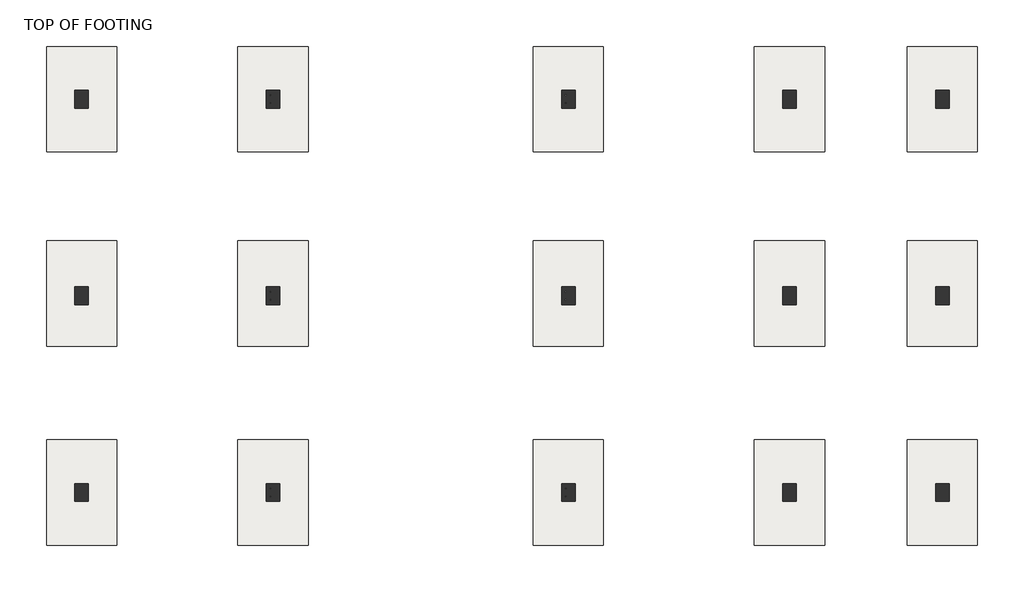
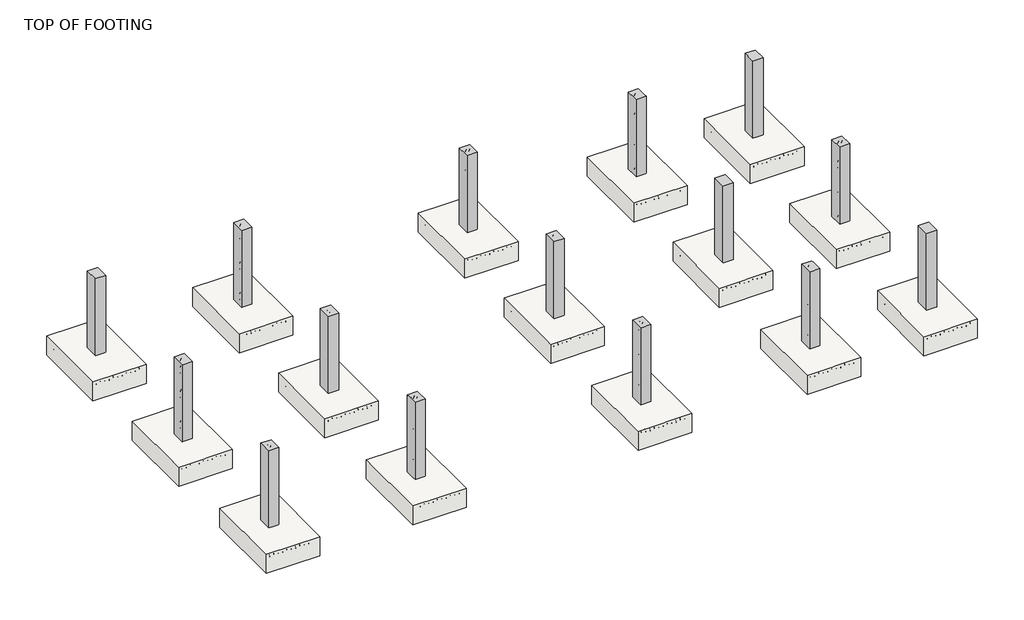
# One storey, part 1 of 8: 15 columns, 15 slabs.
"""IFC4 building model written with IfcOpenShell, lengths in millimetres."""

from ifc_helpers import new_model, si_unit, origin, place, context, project, spatial, faceted_brep, transform, mapped, element, save
from components import m_footing_rectangular_1800_x_1200_x_450mm_16ba7ea5

model = new_model("IFC4")

# Units and contexts
model_context = context("Model", 3, world=origin())
ifc_project = project(units=[si_unit("LENGTHUNIT", "METRE", prefix="MILLI")], contexts=[model_context])

# Site, building, storey
site = spatial("IfcSite", under=ifc_project)
building = spatial("IfcBuilding", under=site)
storey = spatial("IfcBuildingStorey", under=building, Name="TOP OF FOOTING", Elevation=-1828.8)

# Columns
placement = place(None, origin())
element("IfcColumn", 1, ObjectType="M_Concrete-Rectangular-Column : 9\" X 1' COLUMNS", at=placement, inside=storey, context=model_context, shape_type="Brep", body=[
    faceted_brep([(9617.8931183, 9077.6765586, -1828.8), (9617.8931183, 8772.8765586, -1828.8), (9389.2931183, 8772.8765586, -1828.8), (9389.2931183, 9077.6765586, -1828.8), (9617.8931183, 9077.6765586, 0.0), (9617.8931183, 8772.8765586, 0.0), (9389.2931183, 8772.8765586, 0.0), (9389.2931183, 8849.0765586, 0.0), (9389.2931183, 9077.6765586, 0.0)], [[[0, 1, 2, 3]], [[4, 5, 1, 0]], [[5, 6, 2, 1]], [[6, 7, 8, 3, 2]], [[8, 4, 0, 3]], [[4, 8, 7, 6, 5]]]),
])
element("IfcColumn", 2, ObjectType="M_Concrete-Rectangular-Column : 9\" X 1' COLUMNS", at=placement, inside=storey, context=model_context, shape_type="Brep", body=[
    faceted_brep([(9617.8931183, 5712.0180792, -1828.8), (9617.8931183, 5407.2180792, -1828.8), (9389.2931183, 5407.2180792, -1828.8), (9389.2931183, 5712.0180792, -1828.8), (9617.8931183, 5712.0180792, 0.0), (9617.8931183, 5407.2180792, 0.0), (9389.2931183, 5407.2180792, 0.0), (9389.2931183, 5445.3180792, 0.0), (9389.2931183, 5673.9180792, 0.0), (9389.2931183, 5712.0180792, 0.0)], [[[0, 1, 2, 3]], [[4, 5, 1, 0]], [[5, 6, 2, 1]], [[6, 7, 8, 9, 3, 2]], [[9, 4, 0, 3]], [[4, 9, 8, 7, 6, 5]]]),
])
element("IfcColumn", 3, ObjectType="M_Concrete-Rectangular-Column : 9\" X 1' COLUMNS", at=placement, inside=storey, context=model_context, shape_type="Brep", body=[
    faceted_brep([(9617.8931183, 2346.6765586, -1828.8), (9617.8931183, 2041.8765586, -1828.8), (9389.2931183, 2041.8765586, -1828.8), (9389.2931183, 2346.6765586, -1828.8), (9617.8931183, 2346.6765586, 0.0), (9617.8931183, 2041.8765586, 0.0), (9389.2931183, 2041.8765586, 0.0), (9389.2931183, 2270.4765586, 0.0), (9389.2931183, 2346.6765586, 0.0)], [[[0, 1, 2, 3]], [[4, 5, 1, 0]], [[5, 6, 2, 1]], [[6, 7, 8, 3, 2]], [[8, 4, 0, 3]], [[4, 8, 7, 6, 5]]]),
])
element("IfcColumn", 4, ObjectType="M_Concrete-Rectangular-Column : 9\" X 1' COLUMNS", at=placement, inside=storey, context=model_context, shape_type="Brep", body=[
    faceted_brep([(7001.6931183, 9077.6765586, -1828.8), (7001.6931183, 8772.8765586, -1828.8), (6773.0931183, 8772.8765586, -1828.8), (6773.0931183, 9077.6765586, -1828.8), (7001.6931183, 9077.6765586, 0.0), (7001.6931183, 8849.0765586, 0.0), (7001.6931183, 8772.8765586, 0.0), (7001.6931183, 8772.8765586, -300.0), (6773.0931183, 8772.8765586, 0.0), (6773.0931183, 8772.8765586, -300.0), (6773.0931183, 8849.0765586, 0.0), (6773.0931183, 9077.6765586, 0.0)], [[[0, 1, 2, 3]], [[1, 0, 4, 5, 6, 7]], [[2, 1, 7, 6, 8, 9]], [[3, 2, 9, 8, 10, 11]], [[0, 3, 11, 4]], [[8, 6, 5, 4, 11, 10]]]),
])
element("IfcColumn", 5, ObjectType="M_Concrete-Rectangular-Column : 9\" X 1' COLUMNS", at=placement, inside=storey, context=model_context, shape_type="Brep", body=[
    faceted_brep([(7001.6931183, 5712.0180792, -1828.8), (7001.6931183, 5407.2180792, -1828.8), (6773.0931183, 5407.2180792, -1828.8), (6773.0931183, 5712.0180792, -1828.8), (7001.6931183, 5712.0180792, -300.0), (7001.6931183, 5712.0180792, 0.0), (7001.6931183, 5673.9180792, 0.0), (7001.6931183, 5445.3180792, 0.0), (7001.6931183, 5407.2180792, 0.0), (7001.6931183, 5407.2180792, -300.0), (6773.0931183, 5407.2180792, 0.0), (6773.0931183, 5407.2180792, -300.0), (6773.0931183, 5445.3180792, 0.0), (6773.0931183, 5673.9180792, 0.0), (6773.0931183, 5712.0180792, 0.0), (6773.0931183, 5712.0180792, -300.0)], [[[0, 1, 2, 3]], [[1, 0, 4, 5, 6, 7, 8, 9]], [[2, 1, 9, 8, 10, 11]], [[3, 2, 11, 10, 12, 13, 14, 15]], [[0, 3, 15, 14, 5, 4]], [[10, 8, 7, 6, 5, 14, 13, 12]]]),
])
element("IfcColumn", 6, ObjectType="M_Concrete-Rectangular-Column : 9\" X 1' COLUMNS", at=placement, inside=storey, context=model_context, shape_type="Brep", body=[
    faceted_brep([(7001.6931183, 2346.6765586, -1828.8), (7001.6931183, 2041.8765586, -1828.8), (6773.0931183, 2041.8765586, -1828.8), (6773.0931183, 2346.6765586, -1828.8), (7001.6931183, 2346.6765586, -300.0), (7001.6931183, 2346.6765586, 0.0), (7001.6931183, 2270.4765586, 0.0), (7001.6931183, 2041.8765586, 0.0), (6773.0931183, 2041.8765586, 0.0), (6773.0931183, 2270.4765586, 0.0), (6773.0931183, 2346.6765586, 0.0), (6773.0931183, 2346.6765586, -300.0)], [[[0, 1, 2, 3]], [[1, 0, 4, 5, 6, 7]], [[2, 1, 7, 8]], [[3, 2, 8, 9, 10, 11]], [[0, 3, 11, 10, 5, 4]], [[8, 7, 6, 5, 10, 9]]]),
])
element("IfcColumn", 7, ObjectType="M_Concrete-Rectangular-Column : 9\" X 1' COLUMNS", at=placement, inside=storey, context=model_context, shape_type="Brep", body=[
    faceted_brep([(3217.0931183, 9077.6765586, -1828.8), (3217.0931183, 8772.8765586, -1828.8), (2988.4931183, 8772.8765586, -1828.8), (2988.4931183, 9077.6765586, -1828.8), (3217.0931183, 9077.6765586, 0.0), (3217.0931183, 8849.0765586, 0.0), (3217.0931183, 8772.8765586, 0.0), (3217.0931183, 8772.8765586, -300.0), (2988.4931183, 8772.8765586, 0.0), (2988.4931183, 8772.8765586, -300.0), (2988.4931183, 8849.0765586, 0.0), (2988.4931183, 9077.6765586, 0.0)], [[[0, 1, 2, 3]], [[1, 0, 4, 5, 6, 7]], [[2, 1, 7, 6, 8, 9]], [[3, 2, 9, 8, 10, 11]], [[0, 3, 11, 4]], [[8, 6, 5, 4, 11, 10]]]),
])
element("IfcColumn", 8, ObjectType="M_Concrete-Rectangular-Column : 9\" X 1' COLUMNS", at=placement, inside=storey, context=model_context, shape_type="Brep", body=[
    faceted_brep([(3217.0931183, 5712.0180792, -1828.8), (3217.0931183, 5407.2180792, -1828.8), (2988.4931183, 5407.2180792, -1828.8), (2988.4931183, 5712.0180792, -1828.8), (3217.0931183, 5712.0180792, -300.0), (3217.0931183, 5712.0180792, 0.0), (3217.0931183, 5673.9180792, 0.0), (3217.0931183, 5445.3180792, 0.0), (3217.0931183, 5407.2180792, 0.0), (3217.0931183, 5407.2180792, -300.0), (2988.4931183, 5407.2180792, 0.0), (2988.4931183, 5407.2180792, -300.0), (2988.4931183, 5445.3180792, 0.0), (2988.4931183, 5673.9180792, 0.0), (2988.4931183, 5712.0180792, 0.0), (2988.4931183, 5712.0180792, -300.0)], [[[0, 1, 2, 3]], [[1, 0, 4, 5, 6, 7, 8, 9]], [[2, 1, 9, 8, 10, 11]], [[3, 2, 11, 10, 12, 13, 14, 15]], [[0, 3, 15, 14, 5, 4]], [[10, 8, 7, 6, 5, 14, 13, 12]]]),
])
element("IfcColumn", 9, ObjectType="M_Concrete-Rectangular-Column : 9\" X 1' COLUMNS", at=placement, inside=storey, context=model_context, shape_type="Brep", body=[
    faceted_brep([(3217.0931183, 2346.6765586, -1828.8), (3217.0931183, 2041.8765586, -1828.8), (2988.4931183, 2041.8765586, -1828.8), (2988.4931183, 2346.6765586, -1828.8), (3217.0931183, 2346.6765586, -300.0), (3217.0931183, 2346.6765586, 0.0), (3217.0931183, 2270.4765586, 0.0), (3217.0931183, 2041.8765586, 0.0), (2988.4931183, 2041.8765586, 0.0), (2988.4931183, 2270.4765586, 0.0), (2988.4931183, 2346.6765586, 0.0), (2988.4931183, 2346.6765586, -300.0)], [[[0, 1, 2, 3]], [[1, 0, 4, 5, 6, 7]], [[2, 1, 7, 8]], [[3, 2, 8, 9, 10, 11]], [[0, 3, 11, 10, 5, 4]], [[8, 7, 6, 5, 10, 9]]]),
])
element("IfcColumn", 10, ObjectType="M_Concrete-Rectangular-Column : 9\" X 1' COLUMNS", at=placement, inside=storey, context=model_context, shape_type="Brep", body=[
    faceted_brep([(-1837.5068817, 9077.6765586, -1828.8), (-1837.5068817, 8772.8765586, -1828.8), (-2066.1068817, 8772.8765586, -1828.8), (-2066.1068817, 9077.6765586, -1828.8), (-1837.5068817, 9077.6765586, 0.0), (-1837.5068817, 8849.0765586, 0.0), (-1837.5068817, 8810.9765586, 0.0), (-1837.5068817, 8772.8765586, 0.0), (-2066.1068817, 8772.8765586, 0.0), (-2066.1068817, 8772.8765586, -300.0), (-2066.1068817, 8849.0765586, 0.0), (-2066.1068817, 9077.6765586, 0.0)], [[[0, 1, 2, 3]], [[1, 0, 4, 5, 6, 7]], [[2, 1, 7, 8, 9]], [[3, 2, 9, 8, 10, 11]], [[0, 3, 11, 4]], [[8, 7, 6, 5, 4, 11, 10]]]),
])
element("IfcColumn", 11, ObjectType="M_Concrete-Rectangular-Column : 9\" X 1' COLUMNS", at=placement, inside=storey, context=model_context, shape_type="Brep", body=[
    faceted_brep([(-1837.5068817, 5712.0180792, -1828.8), (-1837.5068817, 5407.2180792, -1828.8), (-2066.1068817, 5407.2180792, -1828.8), (-2066.1068817, 5712.0180792, -1828.8), (-1837.5068817, 5712.0180792, -300.0), (-1837.5068817, 5712.0180792, 0.0), (-1837.5068817, 5673.9180792, 0.0), (-1837.5068817, 5445.3180792, 0.0), (-1837.5068817, 5407.2180792, 0.0), (-1837.5068817, 5407.2180792, -300.0), (-2066.1068817, 5407.2180792, 0.0), (-2066.1068817, 5445.3180792, 0.0), (-2066.1068817, 5673.9180792, 0.0), (-2066.1068817, 5712.0180792, 0.0), (-2066.1068817, 5712.0180792, -300.0)], [[[0, 1, 2, 3]], [[1, 0, 4, 5, 6, 7, 8, 9]], [[2, 1, 9, 8, 10]], [[3, 2, 10, 11, 12, 13, 14]], [[0, 3, 14, 13, 5, 4]], [[10, 8, 7, 6, 5, 13, 12, 11]]]),
])
element("IfcColumn", 12, ObjectType="M_Concrete-Rectangular-Column : 9\" X 1' COLUMNS", at=placement, inside=storey, context=model_context, shape_type="Brep", body=[
    faceted_brep([(-1837.5068817, 2346.6765586, -1828.8), (-1837.5068817, 2041.8765586, -1828.8), (-2066.1068817, 2041.8765586, -1828.8), (-2066.1068817, 2346.6765586, -1828.8), (-1837.5068817, 2346.6765586, -300.0), (-1837.5068817, 2346.6765586, 0.0), (-1837.5068817, 2270.4765586, 0.0), (-1837.5068817, 2041.8765586, 0.0), (-2066.1068817, 2041.8765586, 0.0), (-2066.1068817, 2270.4765586, 0.0), (-2066.1068817, 2346.6765586, 0.0)], [[[0, 1, 2, 3]], [[1, 0, 4, 5, 6, 7]], [[2, 1, 7, 8]], [[3, 2, 8, 9, 10]], [[0, 3, 10, 5, 4]], [[8, 7, 6, 5, 10, 9]]]),
])
element("IfcColumn", 13, ObjectType="M_Concrete-Rectangular-Column : 9\" X 1' COLUMNS", at=placement, inside=storey, context=model_context, shape_type="Brep", body=[
    faceted_brep([(-5114.1068817, 2346.6765586, -1828.8), (-5114.1068817, 2041.8765586, -1828.8), (-5342.7068817, 2041.8765586, -1828.8), (-5342.7068817, 2346.6765586, -1828.8), (-5114.1068817, 2346.6765586, 0.0), (-5114.1068817, 2270.4765586, 0.0), (-5114.1068817, 2041.8765586, 0.0), (-5342.7068817, 2041.8765586, 0.0), (-5342.7068817, 2346.6765586, 0.0)], [[[0, 1, 2, 3]], [[4, 5, 6, 1, 0]], [[6, 7, 2, 1]], [[7, 8, 3, 2]], [[8, 4, 0, 3]], [[4, 8, 7, 6, 5]]]),
])
element("IfcColumn", 14, ObjectType="M_Concrete-Rectangular-Column : 9\" X 1' COLUMNS", at=placement, inside=storey, context=model_context, shape_type="Brep", body=[
    faceted_brep([(-5114.1068817, 5712.0180792, -1828.8), (-5114.1068817, 5407.2180792, -1828.8), (-5342.7068817, 5407.2180792, -1828.8), (-5342.7068817, 5712.0180792, -1828.8), (-5114.1068817, 5712.0180792, 0.0), (-5114.1068817, 5673.9180792, 0.0), (-5114.1068817, 5445.3180792, 0.0), (-5114.1068817, 5407.2180792, 0.0), (-5342.7068817, 5407.2180792, 0.0), (-5342.7068817, 5712.0180792, 0.0)], [[[0, 1, 2, 3]], [[4, 5, 6, 7, 1, 0]], [[7, 8, 2, 1]], [[8, 9, 3, 2]], [[9, 4, 0, 3]], [[4, 9, 8, 7, 6, 5]]]),
])
element("IfcColumn", 15, ObjectType="M_Concrete-Rectangular-Column : 9\" X 1' COLUMNS", at=placement, inside=storey, context=model_context, shape_type="Brep", body=[
    faceted_brep([(-5114.1068817, 9077.6765586, -1828.8), (-5114.1068817, 8772.8765586, -1828.8), (-5342.7068817, 8772.8765586, -1828.8), (-5342.7068817, 9077.6765586, -1828.8), (-5114.1068817, 9077.6765586, 0.0), (-5114.1068817, 8849.0765586, 0.0), (-5114.1068817, 8772.8765586, 0.0), (-5342.7068817, 8772.8765586, 0.0), (-5342.7068817, 9077.6765586, 0.0)], [[[0, 1, 2, 3]], [[4, 5, 6, 1, 0]], [[6, 7, 2, 1]], [[7, 8, 3, 2]], [[8, 4, 0, 3]], [[4, 8, 7, 6, 5]]]),
])

# Slabs
m_footing_rectangular_1800_x_1200_x_450mm_shape = m_footing_rectangular_1800_x_1200_x_450mm_16ba7ea5(model_context)
element("IfcSlab", 16, ObjectType="M_Footing-Rectangular : 1800 x 1200 x 450mm", at=placement, inside=storey, context=model_context, shape_type="MappedRepresentation", body=[
    mapped(m_footing_rectangular_1800_x_1200_x_450mm_shape, transform((-5228.4068817, 8925.2765586, -1828.8), x_axis=(1.0, 0.0, 0.0), y_axis=(0.0, 1.0, 0.0), z_axis=(0.0, 0.0, 1.0))),
])
element("IfcSlab", 17, ObjectType="M_Footing-Rectangular : 1800 x 1200 x 450mm", at=placement, inside=storey, context=model_context, shape_type="MappedRepresentation", body=[
    mapped(m_footing_rectangular_1800_x_1200_x_450mm_shape, transform((-1951.8068817, 8925.2765586, -1828.8), x_axis=(1.0, 0.0, 0.0), y_axis=(0.0, 1.0, 0.0), z_axis=(0.0, 0.0, 1.0))),
])
element("IfcSlab", 18, ObjectType="M_Footing-Rectangular : 1800 x 1200 x 450mm", at=placement, inside=storey, context=model_context, shape_type="MappedRepresentation", body=[
    mapped(m_footing_rectangular_1800_x_1200_x_450mm_shape, transform((3102.7931183, 8925.2765586, -1828.8), x_axis=(1.0, 0.0, 0.0), y_axis=(0.0, 1.0, 0.0), z_axis=(0.0, 0.0, 1.0))),
])
element("IfcSlab", 19, ObjectType="M_Footing-Rectangular : 1800 x 1200 x 450mm", at=placement, inside=storey, context=model_context, shape_type="MappedRepresentation", body=[
    mapped(m_footing_rectangular_1800_x_1200_x_450mm_shape, transform((6887.3931183, 8925.2765586, -1828.8), x_axis=(1.0, 0.0, 0.0), y_axis=(0.0, 1.0, 0.0), z_axis=(0.0, 0.0, 1.0))),
])
element("IfcSlab", 20, ObjectType="M_Footing-Rectangular : 1800 x 1200 x 450mm", at=placement, inside=storey, context=model_context, shape_type="MappedRepresentation", body=[
    mapped(m_footing_rectangular_1800_x_1200_x_450mm_shape, transform((9503.5931183, 8925.2765586, -1828.8), x_axis=(1.0, 0.0, 0.0), y_axis=(0.0, 1.0, 0.0), z_axis=(0.0, 0.0, 1.0))),
])
element("IfcSlab", 21, ObjectType="M_Footing-Rectangular : 1800 x 1200 x 450mm", at=placement, inside=storey, context=model_context, shape_type="MappedRepresentation", body=[
    mapped(m_footing_rectangular_1800_x_1200_x_450mm_shape, transform((-5228.4068817, 5598.1162126, -1828.8), x_axis=(1.0, 0.0, 0.0), y_axis=(0.0, 1.0, 0.0), z_axis=(0.0, 0.0, 1.0))),
])
element("IfcSlab", 22, ObjectType="M_Footing-Rectangular : 1800 x 1200 x 450mm", at=placement, inside=storey, context=model_context, shape_type="MappedRepresentation", body=[
    mapped(m_footing_rectangular_1800_x_1200_x_450mm_shape, transform((-1951.8068817, 5598.1162126, -1828.8), x_axis=(1.0, 0.0, 0.0), y_axis=(0.0, 1.0, 0.0), z_axis=(0.0, 0.0, 1.0))),
])
element("IfcSlab", 23, ObjectType="M_Footing-Rectangular : 1800 x 1200 x 450mm", at=placement, inside=storey, context=model_context, shape_type="MappedRepresentation", body=[
    mapped(m_footing_rectangular_1800_x_1200_x_450mm_shape, transform((3102.7931183, 5598.1162126, -1828.8), x_axis=(1.0, 0.0, 0.0), y_axis=(0.0, 1.0, 0.0), z_axis=(0.0, 0.0, 1.0))),
])
element("IfcSlab", 24, ObjectType="M_Footing-Rectangular : 1800 x 1200 x 450mm", at=placement, inside=storey, context=model_context, shape_type="MappedRepresentation", body=[
    mapped(m_footing_rectangular_1800_x_1200_x_450mm_shape, transform((6887.3931183, 5598.1162126, -1828.8), x_axis=(1.0, 0.0, 0.0), y_axis=(0.0, 1.0, 0.0), z_axis=(0.0, 0.0, 1.0))),
])
element("IfcSlab", 25, ObjectType="M_Footing-Rectangular : 1800 x 1200 x 450mm", at=placement, inside=storey, context=model_context, shape_type="MappedRepresentation", body=[
    mapped(m_footing_rectangular_1800_x_1200_x_450mm_shape, transform((9503.5931183, 5598.1162126, -1828.8), x_axis=(1.0, 0.0, 0.0), y_axis=(0.0, 1.0, 0.0), z_axis=(0.0, 0.0, 1.0))),
])
element("IfcSlab", 26, ObjectType="M_Footing-Rectangular : 1800 x 1200 x 450mm", at=placement, inside=storey, context=model_context, shape_type="MappedRepresentation", body=[
    mapped(m_footing_rectangular_1800_x_1200_x_450mm_shape, transform((-5228.4068817, 2194.2765586, -1828.8), x_axis=(1.0, 0.0, 0.0), y_axis=(0.0, 1.0, 0.0), z_axis=(0.0, 0.0, 1.0))),
])
element("IfcSlab", 27, ObjectType="M_Footing-Rectangular : 1800 x 1200 x 450mm", at=placement, inside=storey, context=model_context, shape_type="MappedRepresentation", body=[
    mapped(m_footing_rectangular_1800_x_1200_x_450mm_shape, transform((-1951.8068817, 2194.2765586, -1828.8), x_axis=(1.0, 0.0, 0.0), y_axis=(0.0, 1.0, 0.0), z_axis=(0.0, 0.0, 1.0))),
])
element("IfcSlab", 28, ObjectType="M_Footing-Rectangular : 1800 x 1200 x 450mm", at=placement, inside=storey, context=model_context, shape_type="MappedRepresentation", body=[
    mapped(m_footing_rectangular_1800_x_1200_x_450mm_shape, transform((3102.7931183, 2194.2765586, -1828.8), x_axis=(1.0, 0.0, 0.0), y_axis=(0.0, 1.0, 0.0), z_axis=(0.0, 0.0, 1.0))),
])
element("IfcSlab", 29, ObjectType="M_Footing-Rectangular : 1800 x 1200 x 450mm", at=placement, inside=storey, context=model_context, shape_type="MappedRepresentation", body=[
    mapped(m_footing_rectangular_1800_x_1200_x_450mm_shape, transform((6887.3931183, 2194.2765586, -1828.8), x_axis=(1.0, 0.0, 0.0), y_axis=(0.0, 1.0, 0.0), z_axis=(0.0, 0.0, 1.0))),
])
element("IfcSlab", 30, ObjectType="M_Footing-Rectangular : 1800 x 1200 x 450mm", at=placement, inside=storey, context=model_context, shape_type="MappedRepresentation", body=[
    mapped(m_footing_rectangular_1800_x_1200_x_450mm_shape, transform((9503.5931183, 2194.2765586, -1828.8), x_axis=(1.0, 0.0, 0.0), y_axis=(0.0, 1.0, 0.0), z_axis=(0.0, 0.0, 1.0))),
])

save(model, "model.ifc")

# Revit data of these elements
# Grids (mm)
#   "2": line (-1951.807, -1938.896) -> (-1951.807, 10446.301)
#   "C": line (14910.572, 2194.277) -> (-8013.025, 2194.277)
#   "A": line (12328.531, 8925.277) -> (-8013.025, 8925.277)
#   "4": line (6887.393, 10446.301) -> (6887.393, -2193.704)
#   "5": line (9503.593, -2158.646) -> (9503.593, 10446.301)
#   "B": line (-7983.368, 5605.316) -> (12229.156, 5552.496)
#   "1": line (-5228.407, -1286.673) -> (-5228.407, 10446.301)
#   "3": line (3102.793, -1972.339) -> (3102.793, 10446.301)
# Type "M_Concrete-Rectangular-Column : 9\" X 1' COLUMNS"
#   b = 228.6 mm
#   h = 304.8 mm
#   Structural Material [instance default] = Concrete, Cast-in-Place gray
# Type "M_Footing-Rectangular : 1800 x 1200 x 450mm"
#   Width = 1200 mm
#   Length = 1800 mm
#   Foundation Thickness = 450 mm
#   Structural Material [instance default] = Concrete, Cast-in-Place gray
#   Assembly Code = ""
# Elements 1, 2, 3, 4, 5, 6, 7, 8, 9, 10, 11, 12, 13, 14, 15 (IfcColumn, "M_Concrete-Rectangular-Column : 9\" X 1' COLUMNS")
#   Structural Material = Concrete, Cast-in-Place gray
#   Phase Created = New Construction
#   Materials on its faces: "Concrete, Cast-in-Place gray"
# Elements 16, 17, 18, 19, 20, 21, 22, 23, 24, 25, 26, 27, 28, 29, 30 (IfcSlab, "M_Footing-Rectangular : 1800 x 1200 x 450mm")
#   Structural Material = Concrete, Cast-in-Place gray
#   Phase Created = New Construction
#   Materials on its faces: "Concrete, Cast-in-Place gray"
# Materials
#   "Concrete, Cast-in-Place gray": class "Concrete", colour RGB 192 192 192, transparency 0, Description = "Cast-in-place concrete", Cost = 0
